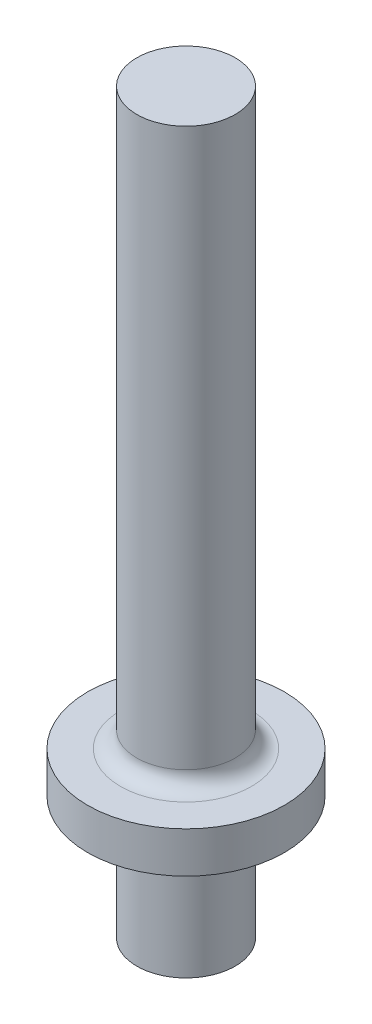
ISO-10303-21;
HEADER;
FILE_DESCRIPTION(('STEP AP214'),'2;1');
FILE_NAME('part.step','',(''),(''),'','','');
FILE_SCHEMA(('AUTOMOTIVE_DESIGN { 1 0 10303 214 1 1 1 1 }'));
ENDSEC;
DATA;
#1=APPLICATION_CONTEXT('core data for automotive mechanical design processes');
#2=APPLICATION_PROTOCOL_DEFINITION('international standard','automotive_design',2000,#1);
#3=PRODUCT_CONTEXT('',#1,'mechanical');
#4=PRODUCT('Part','Part','',(#3));
#5=PRODUCT_RELATED_PRODUCT_CATEGORY('part','',(#4));
#6=PRODUCT_DEFINITION_FORMATION('','',#4);
#7=PRODUCT_DEFINITION_CONTEXT('part definition',#1,'design');
#8=PRODUCT_DEFINITION('design','',#6,#7);
#9=PRODUCT_DEFINITION_SHAPE('','',#8);
#10=(LENGTH_UNIT() NAMED_UNIT(*) SI_UNIT(.MILLI.,.METRE.));
#11=(NAMED_UNIT(*) PLANE_ANGLE_UNIT() SI_UNIT($,.RADIAN.));
#12=(NAMED_UNIT(*) SI_UNIT($,.STERADIAN.) SOLID_ANGLE_UNIT());
#13=UNCERTAINTY_MEASURE_WITH_UNIT(LENGTH_MEASURE(1.E-05),#10,'distance_accuracy_value','');
#14=(GEOMETRIC_REPRESENTATION_CONTEXT(3) GLOBAL_UNCERTAINTY_ASSIGNED_CONTEXT((#13)) GLOBAL_UNIT_ASSIGNED_CONTEXT((#10,
#11,#12)) REPRESENTATION_CONTEXT('',''));
#15=CARTESIAN_POINT('',(0.,0.,0.));
#16=DIRECTION('',(0.,0.,1.));
#17=DIRECTION('',(1.,0.,0.));
#18=AXIS2_PLACEMENT_3D('',#15,#16,#17);
#19=CARTESIAN_POINT('',(0.,0.,0.));
#20=DIRECTION('',(0.,-1.,0.));
#21=DIRECTION('',(0.,0.,-1.));
#22=AXIS2_PLACEMENT_3D('',#19,#20,#21);
#23=PLANE('',#22);
#24=CARTESIAN_POINT('',(0.,0.,0.));
#25=DIRECTION('',(0.,-1.,0.));
#26=DIRECTION('',(0.,0.,-1.));
#27=AXIS2_PLACEMENT_3D('',#24,#25,#26);
#28=CIRCLE('',#27,6.);
#29=CARTESIAN_POINT('',(0.,0.,-6.));
#30=VERTEX_POINT('',#29);
#31=EDGE_CURVE('E48',#30,#30,#28,.T.);
#32=ORIENTED_EDGE('',*,*,#31,.T.);
#33=EDGE_LOOP('',(#32));
#34=FACE_BOUND('',#33,.T.);
#35=ADVANCED_FACE('F40',(#34),#23,.T.);
#36=CARTESIAN_POINT('',(0.,-19.6574585635359,0.));
#37=DIRECTION('',(0.,-1.,0.));
#38=DIRECTION('',(0.,0.,-1.));
#39=AXIS2_PLACEMENT_3D('',#36,#37,#38);
#40=CYLINDRICAL_SURFACE('',#39,6.);
#41=CARTESIAN_POINT('',(0.,15.,0.));
#42=DIRECTION('',(0.,-1.,0.));
#43=DIRECTION('',(0.,0.,-1.));
#44=AXIS2_PLACEMENT_3D('',#41,#42,#43);
#45=CIRCLE('',#44,6.);
#46=CARTESIAN_POINT('',(0.,15.,-6.));
#47=VERTEX_POINT('',#46);
#48=EDGE_CURVE('E55',#47,#47,#45,.T.);
#49=ORIENTED_EDGE('',*,*,#48,.T.);
#50=EDGE_LOOP('',(#49));
#51=FACE_BOUND('',#50,.T.);
#52=ORIENTED_EDGE('',*,*,#31,.F.);
#53=EDGE_LOOP('',(#52));
#54=FACE_BOUND('',#53,.T.);
#55=ADVANCED_FACE('F85',(#51,#54),#40,.T.);
#56=CARTESIAN_POINT('',(6.,15.,0.));
#57=DIRECTION('',(0.,-1.,0.));
#58=DIRECTION('',(0.,0.,-1.));
#59=AXIS2_PLACEMENT_3D('',#56,#57,#58);
#60=PLANE('',#59);
#61=CARTESIAN_POINT('',(0.,15.,0.));
#62=DIRECTION('',(0.,-1.,0.));
#63=DIRECTION('',(0.,0.,-1.));
#64=AXIS2_PLACEMENT_3D('',#61,#62,#63);
#65=CIRCLE('',#64,12.);
#66=CARTESIAN_POINT('',(0.,15.,-12.));
#67=VERTEX_POINT('',#66);
#68=EDGE_CURVE('E60',#67,#67,#65,.T.);
#69=ORIENTED_EDGE('',*,*,#68,.T.);
#70=EDGE_LOOP('',(#69));
#71=FACE_BOUND('',#70,.T.);
#72=ORIENTED_EDGE('',*,*,#48,.F.);
#73=EDGE_LOOP('',(#72));
#74=FACE_BOUND('',#73,.T.);
#75=ADVANCED_FACE('F89',(#71,#74),#60,.T.);
#76=CARTESIAN_POINT('',(0.,-19.6574585635359,0.));
#77=DIRECTION('',(0.,-1.,0.));
#78=DIRECTION('',(0.,0.,-1.));
#79=AXIS2_PLACEMENT_3D('',#76,#77,#78);
#80=CYLINDRICAL_SURFACE('',#79,12.);
#81=CARTESIAN_POINT('',(0.,20.,0.));
#82=DIRECTION('',(0.,-1.,0.));
#83=DIRECTION('',(0.,0.,-1.));
#84=AXIS2_PLACEMENT_3D('',#81,#82,#83);
#85=CIRCLE('',#84,12.);
#86=CARTESIAN_POINT('',(0.,20.,-12.));
#87=VERTEX_POINT('',#86);
#88=EDGE_CURVE('E58',#87,#87,#85,.T.);
#89=ORIENTED_EDGE('',*,*,#88,.T.);
#90=EDGE_LOOP('',(#89));
#91=FACE_BOUND('',#90,.T.);
#92=ORIENTED_EDGE('',*,*,#68,.F.);
#93=EDGE_LOOP('',(#92));
#94=FACE_BOUND('',#93,.T.);
#95=ADVANCED_FACE('F91',(#91,#94),#80,.T.);
#96=CARTESIAN_POINT('',(12.,20.,0.));
#97=DIRECTION('',(0.,1.,0.));
#98=DIRECTION('',(0.,0.,1.));
#99=AXIS2_PLACEMENT_3D('',#96,#97,#98);
#100=PLANE('',#99);
#101=CARTESIAN_POINT('',(0.,20.,0.));
#102=DIRECTION('',(0.,1.,0.));
#103=DIRECTION('',(0.,0.,1.));
#104=AXIS2_PLACEMENT_3D('',#101,#102,#103);
#105=CIRCLE('',#104,8.);
#106=CARTESIAN_POINT('',(0.,20.,8.));
#107=VERTEX_POINT('',#106);
#108=EDGE_CURVE('E42',#107,#107,#105,.F.);
#109=ORIENTED_EDGE('',*,*,#108,.T.);
#110=EDGE_LOOP('',(#109));
#111=FACE_BOUND('',#110,.T.);
#112=ORIENTED_EDGE('',*,*,#88,.F.);
#113=EDGE_LOOP('',(#112));
#114=FACE_BOUND('',#113,.T.);
#115=ADVANCED_FACE('F79',(#111,#114),#100,.T.);
#116=CARTESIAN_POINT('',(0.,-19.6574585635359,0.));
#117=DIRECTION('',(0.,-1.,0.));
#118=DIRECTION('',(0.,0.,-1.));
#119=AXIS2_PLACEMENT_3D('',#116,#117,#118);
#120=CYLINDRICAL_SURFACE('',#119,6.);
#121=CARTESIAN_POINT('',(0.,22.,0.));
#122=DIRECTION('',(0.,1.,0.));
#123=DIRECTION('',(0.,0.,1.));
#124=AXIS2_PLACEMENT_3D('',#121,#122,#123);
#125=CIRCLE('',#124,6.);
#126=CARTESIAN_POINT('',(0.,22.,6.));
#127=VERTEX_POINT('',#126);
#128=EDGE_CURVE('E10',#127,#127,#125,.T.);
#129=ORIENTED_EDGE('',*,*,#128,.T.);
#130=EDGE_LOOP('',(#129));
#131=FACE_BOUND('',#130,.T.);
#132=CARTESIAN_POINT('',(0.,90.,0.));
#133=DIRECTION('',(0.,-1.,0.));
#134=DIRECTION('',(0.,0.,-1.));
#135=AXIS2_PLACEMENT_3D('',#132,#133,#134);
#136=CIRCLE('',#135,6.);
#137=CARTESIAN_POINT('',(0.,90.,-6.));
#138=VERTEX_POINT('',#137);
#139=EDGE_CURVE('E64',#138,#138,#136,.T.);
#140=ORIENTED_EDGE('',*,*,#139,.T.);
#141=EDGE_LOOP('',(#140));
#142=FACE_BOUND('',#141,.T.);
#143=ADVANCED_FACE('F69',(#131,#142),#120,.T.);
#144=CARTESIAN_POINT('',(6.,90.,0.));
#145=DIRECTION('',(0.,1.,0.));
#146=DIRECTION('',(0.,0.,1.));
#147=AXIS2_PLACEMENT_3D('',#144,#145,#146);
#148=PLANE('',#147);
#149=ORIENTED_EDGE('',*,*,#139,.F.);
#150=EDGE_LOOP('',(#149));
#151=FACE_BOUND('',#150,.T.);
#152=ADVANCED_FACE('F66',(#151),#148,.T.);
#153=CARTESIAN_POINT('',(0.,22.,0.));
#154=DIRECTION('',(0.,1.,0.));
#155=DIRECTION('',(0.,0.,1.));
#156=AXIS2_PLACEMENT_3D('',#153,#154,#155);
#157=TOROIDAL_SURFACE('',#156,8.,2.);
#158=ORIENTED_EDGE('',*,*,#128,.F.);
#159=EDGE_LOOP('',(#158));
#160=FACE_BOUND('',#159,.T.);
#161=ORIENTED_EDGE('',*,*,#108,.F.);
#162=EDGE_LOOP('',(#161));
#163=FACE_BOUND('',#162,.T.);
#164=ADVANCED_FACE('F39',(#160,#163),#157,.F.);
#165=CLOSED_SHELL('',(#35,#55,#75,#95,#115,#143,#152,#164));
#166=MANIFOLD_SOLID_BREP('B2',#165);
#167=ADVANCED_BREP_SHAPE_REPRESENTATION('',(#18,#166),#14);
#168=SHAPE_DEFINITION_REPRESENTATION(#9,#167);
ENDSEC;
END-ISO-10303-21;
